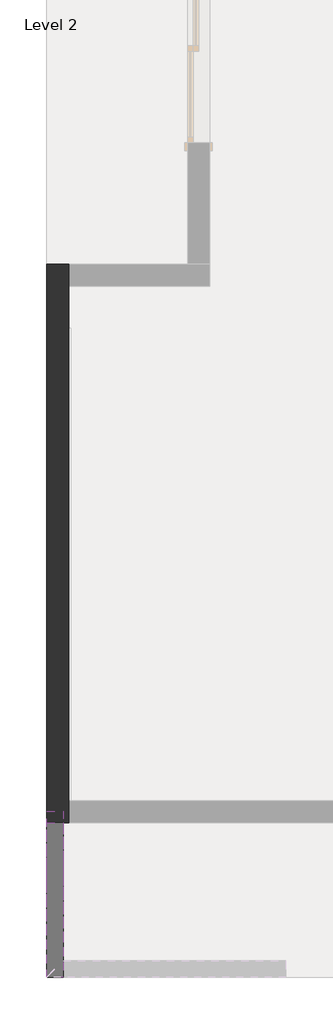
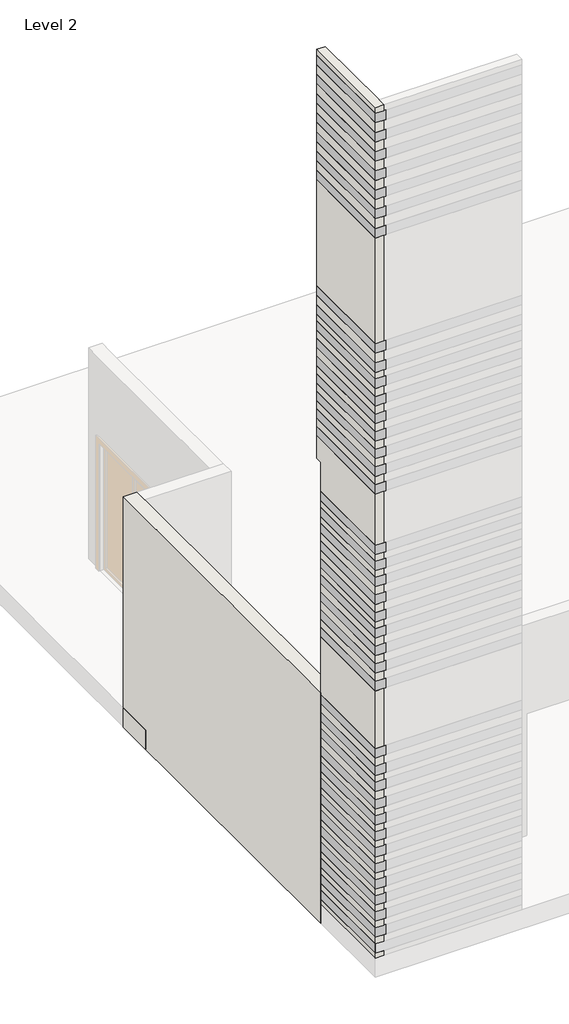
# One storey, part 1 of 2: 38 proxies, 2 walls.
"""IFC4 building model written with IfcOpenShell, lengths in millimetres."""

from ifc_helpers import new_model, si_unit, frame, origin, place, context, project, spatial, polyline, outline, extrude, faceted_brep, element, save

model = new_model("IFC4")

# Units and contexts
model_context = context("Model", 3, world=origin())
ifc_project = project(units=[si_unit("LENGTHUNIT", "METRE", prefix="MILLI")], contexts=[model_context])

# Site, building, storey
site = spatial("IfcSite", under=ifc_project)
building = spatial("IfcBuilding", under=site)
storey = spatial("IfcBuildingStorey", under=building, Name="Level 2", Elevation=3657.6)

# Proxies
placement = place(None, origin())
element("IfcBuildingElementProxy", 1, Name="Reveal", ObjectType="Reveal", at=placement, inside=storey, context=model_context, shape_type="SweptSolid", body=[
    extrude(outline(polyline([(-8860.5727738, -2566.8325754), (-8708.1727738, -2566.8325754), (-8708.1727738, -3836.8325754), (-8860.5727738, -3989.2325754), (-8860.5727738, -2566.8325754)])), frame((0.0, 0.0, 4038.6), z_axis=(0.0, 0.0, 1.0), x_axis=(1.0, 0.0, 0.0)), (0.0, 0.0, 1.0), 152.4),
])
element("IfcBuildingElementProxy", 2, Name="Reveal", ObjectType="Reveal", at=placement, inside=storey, context=model_context, shape_type="SweptSolid", body=[
    extrude(outline(polyline([(-8860.5727738, -2566.8325754), (-8708.1727738, -2566.8325754), (-8708.1727738, -3989.2325754), (-8860.5727738, -3989.2325754), (-8860.5727738, -2566.8325754)])), frame((0.0, 0.0, 4292.6), z_axis=(0.0, 0.0, 1.0), x_axis=(1.0, 0.0, 0.0)), (0.0, 0.0, 1.0), 152.4),
])
element("IfcBuildingElementProxy", 3, Name="Reveal", ObjectType="Reveal", at=placement, inside=storey, context=model_context, shape_type="SweptSolid", body=[
    extrude(outline(polyline([(-8860.5727738, -2566.8325754), (-8708.1727738, -2566.8325754), (-8708.1727738, -3989.2325754), (-8860.5727738, -3989.2325754), (-8860.5727738, -2566.8325754)])), frame((0.0, 0.0, 4546.6), z_axis=(0.0, 0.0, 1.0), x_axis=(1.0, 0.0, 0.0)), (0.0, 0.0, 1.0), 152.4),
])
element("IfcBuildingElementProxy", 4, Name="Reveal", ObjectType="Reveal", at=placement, inside=storey, context=model_context, shape_type="SweptSolid", body=[
    extrude(outline(polyline([(-8860.5727738, -2566.8325754), (-8708.1727738, -2566.8325754), (-8708.1727738, -3989.2325754), (-8860.5727738, -3989.2325754), (-8860.5727738, -2566.8325754)])), frame((0.0, 0.0, 4800.6), z_axis=(0.0, 0.0, 1.0), x_axis=(1.0, 0.0, 0.0)), (0.0, 0.0, 1.0), 152.4),
])
element("IfcBuildingElementProxy", 5, Name="Reveal", ObjectType="Reveal", at=placement, inside=storey, context=model_context, shape_type="SweptSolid", body=[
    extrude(outline(polyline([(-8860.5727738, -2566.8325754), (-8708.1727738, -2566.8325754), (-8708.1727738, -3989.2325754), (-8860.5727738, -3989.2325754), (-8860.5727738, -2566.8325754)])), frame((0.0, 0.0, 5054.6), z_axis=(0.0, 0.0, 1.0), x_axis=(1.0, 0.0, 0.0)), (0.0, 0.0, 1.0), 152.4),
])
element("IfcBuildingElementProxy", 6, Name="Reveal", ObjectType="Reveal", at=placement, inside=storey, context=model_context, shape_type="SweptSolid", body=[
    extrude(outline(polyline([(-8860.5727738, -2566.8325754), (-8708.1727738, -2566.8325754), (-8708.1727738, -3989.2325754), (-8860.5727738, -3989.2325754), (-8860.5727738, -2566.8325754)])), frame((0.0, 0.0, 5308.6), z_axis=(0.0, 0.0, 1.0), x_axis=(1.0, 0.0, 0.0)), (0.0, 0.0, 1.0), 152.4),
])
element("IfcBuildingElementProxy", 7, Name="Reveal", ObjectType="Reveal", at=placement, inside=storey, context=model_context, shape_type="SweptSolid", body=[
    extrude(outline(polyline([(-8860.5727738, -2566.8325754), (-8708.1727738, -2566.8325754), (-8708.1727738, -3989.2325754), (-8860.5727738, -3989.2325754), (-8860.5727738, -2566.8325754)])), frame((0.0, 0.0, 5562.6), z_axis=(0.0, 0.0, 1.0), x_axis=(1.0, 0.0, 0.0)), (0.0, 0.0, 1.0), 152.4),
])
element("IfcBuildingElementProxy", 8, Name="Reveal", ObjectType="Reveal", at=placement, inside=storey, context=model_context, shape_type="SweptSolid", body=[
    extrude(outline(polyline([(-8860.5727738, -2566.8325754), (-8708.1727738, -2566.8325754), (-8708.1727738, -3989.2325754), (-8860.5727738, -3989.2325754), (-8860.5727738, -2566.8325754)])), frame((0.0, 0.0, 5816.6), z_axis=(0.0, 0.0, 1.0), x_axis=(1.0, 0.0, 0.0)), (0.0, 0.0, 1.0), 152.4),
])
element("IfcBuildingElementProxy", 9, Name="Reveal", ObjectType="Reveal", at=placement, inside=storey, context=model_context, shape_type="SweptSolid", body=[
    extrude(outline(polyline([(-8860.5727738, -2566.8325754), (-8708.1727738, -2566.8325754), (-8708.1727738, -3989.2325754), (-8860.5727738, -3989.2325754), (-8860.5727738, -2566.8325754)])), frame((0.0, 0.0, 6070.6), z_axis=(0.0, 0.0, 1.0), x_axis=(1.0, 0.0, 0.0)), (0.0, 0.0, 1.0), 152.4),
])
element("IfcBuildingElementProxy", 10, Name="Reveal", ObjectType="Reveal", at=placement, inside=storey, context=model_context, shape_type="SweptSolid", body=[
    extrude(outline(polyline([(-8860.5727738, -2566.8325754), (-8708.1727738, -2566.8325754), (-8708.1727738, -3989.2325754), (-8860.5727738, -3989.2325754), (-8860.5727738, -2566.8325754)])), frame((0.0, 0.0, 6324.6), z_axis=(0.0, 0.0, 1.0), x_axis=(1.0, 0.0, 0.0)), (0.0, 0.0, 1.0), 152.4),
])
element("IfcBuildingElementProxy", 11, Name="Reveal", ObjectType="Reveal", at=placement, inside=storey, context=model_context, shape_type="SweptSolid", body=[
    extrude(outline(polyline([(-8860.5727738, -2566.8325754), (-8708.1727738, -2566.8325754), (-8708.1727738, -3989.2325754), (-8860.5727738, -3989.2325754), (-8860.5727738, -2566.8325754)])), frame((0.0, 0.0, 6604.0), z_axis=(0.0, 0.0, 1.0), x_axis=(1.0, 0.0, 0.0)), (0.0, 0.0, 1.0), 152.4),
])
element("IfcBuildingElementProxy", 12, Name="Reveal", ObjectType="Reveal", at=placement, inside=storey, context=model_context, shape_type="SweptSolid", body=[
    extrude(outline(polyline([(-8860.5727738, -2566.8325754), (-8708.1727738, -2566.8325754), (-8708.1727738, -3989.2325754), (-8860.5727738, -3989.2325754), (-8860.5727738, -2566.8325754)])), frame((0.0, 0.0, 6858.0), z_axis=(0.0, 0.0, 1.0), x_axis=(1.0, 0.0, 0.0)), (0.0, 0.0, 1.0), 152.4),
])
element("IfcBuildingElementProxy", 13, Name="Reveal", ObjectType="Reveal", at=placement, inside=storey, context=model_context, shape_type="SweptSolid", body=[
    extrude(outline(polyline([(-8860.5727738, -2566.8325754), (-8708.1727738, -2566.8325754), (-8708.1727738, -3989.2325754), (-8860.5727738, -3989.2325754), (-8860.5727738, -2566.8325754)])), frame((0.0, 0.0, 7137.4), z_axis=(0.0, 0.0, 1.0), x_axis=(1.0, 0.0, 0.0)), (0.0, 0.0, 1.0), 152.4),
])
element("IfcBuildingElementProxy", 14, Name="Reveal", ObjectType="Reveal", at=placement, inside=storey, context=model_context, shape_type="SweptSolid", body=[
    extrude(outline(polyline([(-8860.5727738, -2566.8325754), (-8708.1727738, -2566.8325754), (-8708.1727738, -3989.2325754), (-8860.5727738, -3989.2325754), (-8860.5727738, -2566.8325754)])), frame((0.0, 0.0, 8204.2), z_axis=(0.0, 0.0, 1.0), x_axis=(1.0, 0.0, 0.0)), (0.0, 0.0, 1.0), 152.4),
])
element("IfcBuildingElementProxy", 15, Name="Reveal", ObjectType="Reveal", at=placement, inside=storey, context=model_context, shape_type="SweptSolid", body=[
    extrude(outline(polyline([(-8860.5727738, -2566.8325754), (-8708.1727738, -2566.8325754), (-8708.1727738, -3989.2325754), (-8860.5727738, -3989.2325754), (-8860.5727738, -2566.8325754)])), frame((0.0, 0.0, 8483.6), z_axis=(0.0, 0.0, 1.0), x_axis=(1.0, 0.0, 0.0)), (0.0, 0.0, 1.0), 152.4),
])
element("IfcBuildingElementProxy", 16, Name="Reveal", ObjectType="Reveal", at=placement, inside=storey, context=model_context, shape_type="SweptSolid", body=[
    extrude(outline(polyline([(-8860.5727738, -2566.8325754), (-8708.1727738, -2566.8325754), (-8708.1727738, -3989.2325754), (-8860.5727738, -3989.2325754), (-8860.5727738, -2566.8325754)])), frame((0.0, 0.0, 8763.0), z_axis=(0.0, 0.0, 1.0), x_axis=(1.0, 0.0, 0.0)), (0.0, 0.0, 1.0), 152.4),
])
element("IfcBuildingElementProxy", 17, Name="Reveal", ObjectType="Reveal", at=placement, inside=storey, context=model_context, shape_type="SweptSolid", body=[
    extrude(outline(polyline([(-8860.5727738, -2566.8325754), (-8708.1727738, -2566.8325754), (-8708.1727738, -3989.2325754), (-8860.5727738, -3989.2325754), (-8860.5727738, -2566.8325754)])), frame((0.0, 0.0, 9042.4), z_axis=(0.0, 0.0, 1.0), x_axis=(1.0, 0.0, 0.0)), (0.0, 0.0, 1.0), 152.4),
])
element("IfcBuildingElementProxy", 18, Name="Reveal", ObjectType="Reveal", at=placement, inside=storey, context=model_context, shape_type="SweptSolid", body=[
    extrude(outline(polyline([(-8860.5727738, -2566.8325754), (-8708.1727738, -2566.8325754), (-8708.1727738, -3989.2325754), (-8860.5727738, -3989.2325754), (-8860.5727738, -2566.8325754)])), frame((0.0, 0.0, 9296.4), z_axis=(0.0, 0.0, 1.0), x_axis=(1.0, 0.0, 0.0)), (0.0, 0.0, 1.0), 152.4),
])
element("IfcBuildingElementProxy", 19, Name="Reveal", ObjectType="Reveal", at=placement, inside=storey, context=model_context, shape_type="SweptSolid", body=[
    extrude(outline(polyline([(-8860.5727738, -2566.8325754), (-8708.1727738, -2566.8325754), (-8708.1727738, -3989.2325754), (-8860.5727738, -3989.2325754), (-8860.5727738, -2566.8325754)])), frame((0.0, 0.0, 9575.8), z_axis=(0.0, 0.0, 1.0), x_axis=(1.0, 0.0, 0.0)), (0.0, 0.0, 1.0), 152.4),
])
element("IfcBuildingElementProxy", 20, Name="Reveal", ObjectType="Reveal", at=placement, inside=storey, context=model_context, shape_type="SweptSolid", body=[
    extrude(outline(polyline([(-8860.5727738, -2566.8325754), (-8708.1727738, -2566.8325754), (-8708.1727738, -3989.2325754), (-8860.5727738, -3989.2325754), (-8860.5727738, -2566.8325754)])), frame((0.0, 0.0, 9855.2), z_axis=(0.0, 0.0, 1.0), x_axis=(1.0, 0.0, 0.0)), (0.0, 0.0, 1.0), 152.4),
])
element("IfcBuildingElementProxy", 21, Name="Reveal", ObjectType="Reveal", at=placement, inside=storey, context=model_context, shape_type="SweptSolid", body=[
    extrude(outline(polyline([(-8860.5727738, -2566.8325754), (-8708.1727738, -2566.8325754), (-8708.1727738, -3989.2325754), (-8860.5727738, -3989.2325754), (-8860.5727738, -2566.8325754)])), frame((0.0, 0.0, 10109.2), z_axis=(0.0, 0.0, 1.0), x_axis=(1.0, 0.0, 0.0)), (0.0, 0.0, 1.0), 152.4),
])
element("IfcBuildingElementProxy", 22, Name="Reveal", ObjectType="Reveal", at=placement, inside=storey, context=model_context, shape_type="SweptSolid", body=[
    extrude(outline(polyline([(-8860.5727738, -2566.8325754), (-8708.1727738, -2566.8325754), (-8708.1727738, -3989.2325754), (-8860.5727738, -3989.2325754), (-8860.5727738, -2566.8325754)])), frame((0.0, 0.0, 10363.2), z_axis=(0.0, 0.0, 1.0), x_axis=(1.0, 0.0, 0.0)), (0.0, 0.0, 1.0), 152.4),
])
element("IfcBuildingElementProxy", 23, Name="Reveal", ObjectType="Reveal", at=placement, inside=storey, context=model_context, shape_type="SweptSolid", body=[
    extrude(outline(polyline([(-8860.5727738, -2465.2325754), (-8708.1727738, -2465.2325754), (-8708.1727738, -3989.2325754), (-8860.5727738, -3989.2325754), (-8860.5727738, -2465.2325754)])), frame((0.0, 0.0, 11328.4), z_axis=(0.0, 0.0, 1.0), x_axis=(1.0, 0.0, 0.0)), (0.0, 0.0, 1.0), 152.4),
])
element("IfcBuildingElementProxy", 24, Name="Reveal", ObjectType="Reveal", at=placement, inside=storey, context=model_context, shape_type="SweptSolid", body=[
    extrude(outline(polyline([(-8860.5727738, -2465.2325754), (-8708.1727738, -2465.2325754), (-8708.1727738, -3989.2325754), (-8860.5727738, -3989.2325754), (-8860.5727738, -2465.2325754)])), frame((0.0, 0.0, 11607.8), z_axis=(0.0, 0.0, 1.0), x_axis=(1.0, 0.0, 0.0)), (0.0, 0.0, 1.0), 152.4),
])
element("IfcBuildingElementProxy", 25, Name="Reveal", ObjectType="Reveal", at=placement, inside=storey, context=model_context, shape_type="SweptSolid", body=[
    extrude(outline(polyline([(-8860.5727738, -2465.2325754), (-8708.1727738, -2465.2325754), (-8708.1727738, -3989.2325754), (-8860.5727738, -3989.2325754), (-8860.5727738, -2465.2325754)])), frame((0.0, 0.0, 11887.2), z_axis=(0.0, 0.0, 1.0), x_axis=(1.0, 0.0, 0.0)), (0.0, 0.0, 1.0), 152.4),
])
element("IfcBuildingElementProxy", 26, Name="Reveal", ObjectType="Reveal", at=placement, inside=storey, context=model_context, shape_type="SweptSolid", body=[
    extrude(outline(polyline([(-8860.5727738, -2465.2325754), (-8708.1727738, -2465.2325754), (-8708.1727738, -3989.2325754), (-8860.5727738, -3989.2325754), (-8860.5727738, -2465.2325754)])), frame((0.0, 0.0, 12166.6), z_axis=(0.0, 0.0, 1.0), x_axis=(1.0, 0.0, 0.0)), (0.0, 0.0, 1.0), 152.4),
])
element("IfcBuildingElementProxy", 27, Name="Reveal", ObjectType="Reveal", at=placement, inside=storey, context=model_context, shape_type="SweptSolid", body=[
    extrude(outline(polyline([(-8860.5727738, -2465.2325754), (-8708.1727738, -2465.2325754), (-8708.1727738, -3989.2325754), (-8860.5727738, -3989.2325754), (-8860.5727738, -2465.2325754)])), frame((0.0, 0.0, 12446.0), z_axis=(0.0, 0.0, 1.0), x_axis=(1.0, 0.0, 0.0)), (0.0, 0.0, 1.0), 152.4),
])
element("IfcBuildingElementProxy", 28, Name="Reveal", ObjectType="Reveal", at=placement, inside=storey, context=model_context, shape_type="SweptSolid", body=[
    extrude(outline(polyline([(-8860.5727738, -2465.2325754), (-8708.1727738, -2465.2325754), (-8708.1727738, -3989.2325754), (-8860.5727738, -3989.2325754), (-8860.5727738, -2465.2325754)])), frame((0.0, 0.0, 12725.4), z_axis=(0.0, 0.0, 1.0), x_axis=(1.0, 0.0, 0.0)), (0.0, 0.0, 1.0), 152.4),
])
element("IfcBuildingElementProxy", 29, Name="Reveal", ObjectType="Reveal", at=placement, inside=storey, context=model_context, shape_type="SweptSolid", body=[
    extrude(outline(polyline([(-8860.5727738, -2465.2325754), (-8708.1727738, -2465.2325754), (-8708.1727738, -3989.2325754), (-8860.5727738, -3989.2325754), (-8860.5727738, -2465.2325754)])), frame((0.0, 0.0, 13004.8), z_axis=(0.0, 0.0, 1.0), x_axis=(1.0, 0.0, 0.0)), (0.0, 0.0, 1.0), 152.4),
])
element("IfcBuildingElementProxy", 30, Name="Reveal", ObjectType="Reveal", at=placement, inside=storey, context=model_context, shape_type="SweptSolid", body=[
    extrude(outline(polyline([(-8860.5727738, -2465.2325754), (-8708.1727738, -2465.2325754), (-8708.1727738, -3989.2325754), (-8860.5727738, -3989.2325754), (-8860.5727738, -2465.2325754)])), frame((0.0, 0.0, 13258.8), z_axis=(0.0, 0.0, 1.0), x_axis=(1.0, 0.0, 0.0)), (0.0, 0.0, 1.0), 152.4),
])
element("IfcBuildingElementProxy", 31, Name="Reveal", ObjectType="Reveal", at=placement, inside=storey, context=model_context, shape_type="SweptSolid", body=[
    extrude(outline(polyline([(-8860.5727738, -2465.2325754), (-8708.1727738, -2465.2325754), (-8708.1727738, -3989.2325754), (-8860.5727738, -3989.2325754), (-8860.5727738, -2465.2325754)])), frame((0.0, 0.0, 13563.6), z_axis=(0.0, 0.0, 1.0), x_axis=(1.0, 0.0, 0.0)), (0.0, 0.0, 1.0), 152.4),
])
element("IfcBuildingElementProxy", 32, Name="Reveal", ObjectType="Reveal", at=placement, inside=storey, context=model_context, shape_type="SweptSolid", body=[
    extrude(outline(polyline([(-8860.5727738, -2465.2325754), (-8708.1727738, -2465.2325754), (-8708.1727738, -3989.2325754), (-8860.5727738, -3989.2325754), (-8860.5727738, -2465.2325754)])), frame((0.0, 0.0, 15392.4), z_axis=(0.0, 0.0, 1.0), x_axis=(1.0, 0.0, 0.0)), (0.0, 0.0, 1.0), 152.4),
])
element("IfcBuildingElementProxy", 33, Name="Reveal", ObjectType="Reveal", at=placement, inside=storey, context=model_context, shape_type="SweptSolid", body=[
    extrude(outline(polyline([(-8860.5727738, -2465.2325754), (-8708.1727738, -2465.2325754), (-8708.1727738, -3989.2325754), (-8860.5727738, -3989.2325754), (-8860.5727738, -2465.2325754)])), frame((0.0, 0.0, 15697.2), z_axis=(0.0, 0.0, 1.0), x_axis=(1.0, 0.0, 0.0)), (0.0, 0.0, 1.0), 152.4),
])
element("IfcBuildingElementProxy", 34, Name="Reveal", ObjectType="Reveal", at=placement, inside=storey, context=model_context, shape_type="SweptSolid", body=[
    extrude(outline(polyline([(-8860.5727738, -2465.2325754), (-8708.1727738, -2465.2325754), (-8708.1727738, -3989.2325754), (-8860.5727738, -3989.2325754), (-8860.5727738, -2465.2325754)])), frame((0.0, 0.0, 16002.0), z_axis=(0.0, 0.0, 1.0), x_axis=(1.0, 0.0, 0.0)), (0.0, 0.0, 1.0), 152.4),
])
element("IfcBuildingElementProxy", 35, Name="Reveal", ObjectType="Reveal", at=placement, inside=storey, context=model_context, shape_type="SweptSolid", body=[
    extrude(outline(polyline([(-8860.5727738, -2465.2325754), (-8708.1727738, -2465.2325754), (-8708.1727738, -3989.2325754), (-8860.5727738, -3989.2325754), (-8860.5727738, -2465.2325754)])), frame((0.0, 0.0, 16306.8), z_axis=(0.0, 0.0, 1.0), x_axis=(1.0, 0.0, 0.0)), (0.0, 0.0, 1.0), 152.4),
])
element("IfcBuildingElementProxy", 36, Name="Reveal", ObjectType="Reveal", at=placement, inside=storey, context=model_context, shape_type="SweptSolid", body=[
    extrude(outline(polyline([(-8860.5727738, -2465.2325754), (-8708.1727738, -2465.2325754), (-8708.1727738, -3989.2325754), (-8860.5727738, -3989.2325754), (-8860.5727738, -2465.2325754)])), frame((0.0, 0.0, 16611.6), z_axis=(0.0, 0.0, 1.0), x_axis=(1.0, 0.0, 0.0)), (0.0, 0.0, 1.0), 152.4),
])
element("IfcBuildingElementProxy", 37, Name="Reveal", ObjectType="Reveal", at=placement, inside=storey, context=model_context, shape_type="SweptSolid", body=[
    extrude(outline(polyline([(-8860.5727738, -2465.2325754), (-8708.1727738, -2465.2325754), (-8708.1727738, -3989.2325754), (-8860.5727738, -3989.2325754), (-8860.5727738, -2465.2325754)])), frame((0.0, 0.0, 16916.4), z_axis=(0.0, 0.0, 1.0), x_axis=(1.0, 0.0, 0.0)), (0.0, 0.0, 1.0), 152.4),
])
element("IfcBuildingElementProxy", 38, Name="Reveal", ObjectType="Reveal", at=placement, inside=storey, context=model_context, shape_type="SweptSolid", body=[
    extrude(outline(polyline([(-8860.5727738, -2465.2325754), (-8708.1727738, -2465.2325754), (-8708.1727738, -3989.2325754), (-8860.5727738, -3989.2325754), (-8860.5727738, -2465.2325754)])), frame((0.0, 0.0, 17221.2), z_axis=(0.0, 0.0, 1.0), x_axis=(1.0, 0.0, 0.0)), (0.0, 0.0, 1.0), 152.4),
])

# Walls
element("IfcWall", 39, ObjectType="Generic - 5\"", at=placement, inside=storey, context=model_context, shape_type="Brep", body=[
    faceted_brep([(-8860.5727738, -2566.8325754, 3962.4), (-8860.5727738, -3989.2325754, 3962.4), (-8860.5727738, -3989.2325754, 4038.6), (-8860.5727738, -2566.8325754, 4038.6), (-8733.5727738, -3989.2325754, 3962.4), (-8733.5727738, -3862.2325754, 3962.4), (-8733.5727738, -2566.8325754, 3962.4), (-8733.5727738, -2566.8325754, 4038.6), (-8733.5727738, -3862.2325754, 4038.6), (-8733.5727738, -3989.2325754, 4038.6)], [[[0, 1, 2, 3]], [[4, 5, 6, 7, 8, 9]], [[1, 0, 6, 5, 4]], [[1, 4, 9, 2]], [[6, 0, 3, 7]], [[3, 2, 9, 8, 7]]]),
    faceted_brep([(-8860.5727738, -3989.2325754, 17464.824337), (-8860.5727738, -2465.2325754, 17464.824337), (-8860.5727738, -2465.2325754, 17373.6), (-8860.5727738, -3989.2325754, 17373.6), (-8733.5727738, -2465.2325754, 17464.824337), (-8733.5727738, -3862.2325754, 17464.824337), (-8733.5727738, -3989.2325754, 17464.824337), (-8733.5727738, -3989.2325754, 17373.6), (-8733.5727738, -3862.2325754, 17373.6), (-8733.5727738, -2465.2325754, 17373.6)], [[[0, 1, 2, 3]], [[4, 5, 6, 7, 8, 9]], [[1, 0, 6, 5, 4]], [[6, 0, 3, 7]], [[1, 4, 9, 2]], [[3, 2, 9, 8, 7]]]),
    faceted_brep([(-8860.5727738, -2465.2325754, 10972.8), (-8860.5727738, -2566.8325754, 10972.8), (-8860.5727738, -2566.8325754, 10515.6), (-8860.5727738, -3989.2325754, 10515.6), (-8860.5727738, -3989.2325754, 11328.4), (-8860.5727738, -2465.2325754, 11328.4), (-8733.5727738, -2566.8325754, 10972.8), (-8733.5727738, -2509.6825754, 10972.8), (-8733.5727738, -2465.2325754, 10972.8), (-8733.5727738, -2465.2325754, 11328.4), (-8733.5727738, -2509.6825754, 11328.4), (-8733.5727738, -3862.2325754, 11328.4), (-8733.5727738, -3989.2325754, 11328.4), (-8733.5727738, -3989.2325754, 10515.6), (-8733.5727738, -3862.2325754, 10515.6), (-8733.5727738, -2566.8325754, 10515.6)], [[[0, 1, 2, 3, 4, 5]], [[6, 7, 8, 9, 10, 11, 12, 13, 14, 15]], [[3, 13, 12, 4]], [[8, 0, 5, 9]], [[0, 8, 7, 6, 1]], [[1, 6, 15, 2]], [[3, 2, 15, 14, 13]], [[5, 4, 12, 11, 10, 9]]]),
    faceted_brep([(-8860.5727738, -2566.8325754, 4191.0), (-8860.5727738, -3989.2325754, 4191.0), (-8860.5727738, -3989.2325754, 4292.6), (-8860.5727738, -2566.8325754, 4292.6), (-8733.5727738, -3989.2325754, 4191.0), (-8733.5727738, -3862.2325754, 4191.0), (-8733.5727738, -2566.8325754, 4191.0), (-8733.5727738, -2566.8325754, 4292.6), (-8733.5727738, -3862.2325754, 4292.6), (-8733.5727738, -3989.2325754, 4292.6)], [[[0, 1, 2, 3]], [[4, 5, 6, 7, 8, 9]], [[1, 4, 9, 2]], [[6, 0, 3, 7]], [[1, 0, 6, 5, 4]], [[3, 2, 9, 8, 7]]]),
    faceted_brep([(-8860.5727738, -2566.8325754, 4445.0), (-8860.5727738, -3989.2325754, 4445.0), (-8860.5727738, -3989.2325754, 4546.6), (-8860.5727738, -2566.8325754, 4546.6), (-8733.5727738, -3989.2325754, 4445.0), (-8733.5727738, -3862.2325754, 4445.0), (-8733.5727738, -2566.8325754, 4445.0), (-8733.5727738, -2566.8325754, 4546.6), (-8733.5727738, -3862.2325754, 4546.6), (-8733.5727738, -3989.2325754, 4546.6)], [[[0, 1, 2, 3]], [[4, 5, 6, 7, 8, 9]], [[1, 4, 9, 2]], [[6, 0, 3, 7]], [[1, 0, 6, 5, 4]], [[3, 2, 9, 8, 7]]]),
    faceted_brep([(-8860.5727738, -2566.8325754, 4699.0), (-8860.5727738, -3989.2325754, 4699.0), (-8860.5727738, -3989.2325754, 4800.6), (-8860.5727738, -2566.8325754, 4800.6), (-8733.5727738, -3989.2325754, 4699.0), (-8733.5727738, -3862.2325754, 4699.0), (-8733.5727738, -2566.8325754, 4699.0), (-8733.5727738, -2566.8325754, 4800.6), (-8733.5727738, -3862.2325754, 4800.6), (-8733.5727738, -3989.2325754, 4800.6)], [[[0, 1, 2, 3]], [[4, 5, 6, 7, 8, 9]], [[1, 4, 9, 2]], [[6, 0, 3, 7]], [[1, 0, 6, 5, 4]], [[3, 2, 9, 8, 7]]]),
    faceted_brep([(-8860.5727738, -2566.8325754, 4953.0), (-8860.5727738, -3989.2325754, 4953.0), (-8860.5727738, -3989.2325754, 5054.6), (-8860.5727738, -2566.8325754, 5054.6), (-8733.5727738, -3989.2325754, 4953.0), (-8733.5727738, -3862.2325754, 4953.0), (-8733.5727738, -2566.8325754, 4953.0), (-8733.5727738, -2566.8325754, 5054.6), (-8733.5727738, -3862.2325754, 5054.6), (-8733.5727738, -3989.2325754, 5054.6)], [[[0, 1, 2, 3]], [[4, 5, 6, 7, 8, 9]], [[1, 4, 9, 2]], [[6, 0, 3, 7]], [[1, 0, 6, 5, 4]], [[3, 2, 9, 8, 7]]]),
    faceted_brep([(-8860.5727738, -2566.8325754, 5207.0), (-8860.5727738, -3989.2325754, 5207.0), (-8860.5727738, -3989.2325754, 5308.6), (-8860.5727738, -2566.8325754, 5308.6), (-8733.5727738, -3989.2325754, 5207.0), (-8733.5727738, -3862.2325754, 5207.0), (-8733.5727738, -2566.8325754, 5207.0), (-8733.5727738, -2566.8325754, 5308.6), (-8733.5727738, -3862.2325754, 5308.6), (-8733.5727738, -3989.2325754, 5308.6)], [[[0, 1, 2, 3]], [[4, 5, 6, 7, 8, 9]], [[1, 4, 9, 2]], [[6, 0, 3, 7]], [[1, 0, 6, 5, 4]], [[3, 2, 9, 8, 7]]]),
    faceted_brep([(-8860.5727738, -2566.8325754, 5461.0), (-8860.5727738, -3989.2325754, 5461.0), (-8860.5727738, -3989.2325754, 5562.6), (-8860.5727738, -2566.8325754, 5562.6), (-8733.5727738, -3989.2325754, 5461.0), (-8733.5727738, -3862.2325754, 5461.0), (-8733.5727738, -2566.8325754, 5461.0), (-8733.5727738, -2566.8325754, 5562.6), (-8733.5727738, -3862.2325754, 5562.6), (-8733.5727738, -3989.2325754, 5562.6)], [[[0, 1, 2, 3]], [[4, 5, 6, 7, 8, 9]], [[1, 4, 9, 2]], [[6, 0, 3, 7]], [[1, 0, 6, 5, 4]], [[3, 2, 9, 8, 7]]]),
    faceted_brep([(-8860.5727738, -2566.8325754, 5715.0), (-8860.5727738, -3989.2325754, 5715.0), (-8860.5727738, -3989.2325754, 5816.6), (-8860.5727738, -2566.8325754, 5816.6), (-8733.5727738, -3989.2325754, 5715.0), (-8733.5727738, -3862.2325754, 5715.0), (-8733.5727738, -2566.8325754, 5715.0), (-8733.5727738, -2566.8325754, 5816.6), (-8733.5727738, -3862.2325754, 5816.6), (-8733.5727738, -3989.2325754, 5816.6)], [[[0, 1, 2, 3]], [[4, 5, 6, 7, 8, 9]], [[1, 4, 9, 2]], [[6, 0, 3, 7]], [[1, 0, 6, 5, 4]], [[3, 2, 9, 8, 7]]]),
    faceted_brep([(-8860.5727738, -2566.8325754, 5969.0), (-8860.5727738, -3989.2325754, 5969.0), (-8860.5727738, -3989.2325754, 6070.6), (-8860.5727738, -2566.8325754, 6070.6), (-8733.5727738, -3989.2325754, 5969.0), (-8733.5727738, -3862.2325754, 5969.0), (-8733.5727738, -2566.8325754, 5969.0), (-8733.5727738, -2566.8325754, 6070.6), (-8733.5727738, -3862.2325754, 6070.6), (-8733.5727738, -3989.2325754, 6070.6)], [[[0, 1, 2, 3]], [[4, 5, 6, 7, 8, 9]], [[1, 4, 9, 2]], [[6, 0, 3, 7]], [[1, 0, 6, 5, 4]], [[3, 2, 9, 8, 7]]]),
    faceted_brep([(-8860.5727738, -2566.8325754, 6223.0), (-8860.5727738, -3989.2325754, 6223.0), (-8860.5727738, -3989.2325754, 6324.6), (-8860.5727738, -2566.8325754, 6324.6), (-8733.5727738, -3989.2325754, 6223.0), (-8733.5727738, -3862.2325754, 6223.0), (-8733.5727738, -2566.8325754, 6223.0), (-8733.5727738, -2566.8325754, 6324.6), (-8733.5727738, -3862.2325754, 6324.6), (-8733.5727738, -3989.2325754, 6324.6)], [[[0, 1, 2, 3]], [[4, 5, 6, 7, 8, 9]], [[1, 4, 9, 2]], [[6, 0, 3, 7]], [[1, 0, 6, 5, 4]], [[3, 2, 9, 8, 7]]]),
    faceted_brep([(-8860.5727738, -2566.8325754, 6477.0), (-8860.5727738, -3989.2325754, 6477.0), (-8860.5727738, -3989.2325754, 6604.0), (-8860.5727738, -2566.8325754, 6604.0), (-8733.5727738, -3989.2325754, 6477.0), (-8733.5727738, -3862.2325754, 6477.0), (-8733.5727738, -2566.8325754, 6477.0), (-8733.5727738, -2566.8325754, 6604.0), (-8733.5727738, -3862.2325754, 6604.0), (-8733.5727738, -3989.2325754, 6604.0)], [[[0, 1, 2, 3]], [[4, 5, 6, 7, 8, 9]], [[1, 4, 9, 2]], [[6, 0, 3, 7]], [[1, 0, 6, 5, 4]], [[3, 2, 9, 8, 7]]]),
    faceted_brep([(-8860.5727738, -2566.8325754, 6756.4), (-8860.5727738, -3989.2325754, 6756.4), (-8860.5727738, -3989.2325754, 6858.0), (-8860.5727738, -2566.8325754, 6858.0), (-8733.5727738, -3989.2325754, 6756.4), (-8733.5727738, -3862.2325754, 6756.4), (-8733.5727738, -2566.8325754, 6756.4), (-8733.5727738, -2566.8325754, 6858.0), (-8733.5727738, -3862.2325754, 6858.0), (-8733.5727738, -3989.2325754, 6858.0)], [[[0, 1, 2, 3]], [[4, 5, 6, 7, 8, 9]], [[1, 4, 9, 2]], [[6, 0, 3, 7]], [[1, 0, 6, 5, 4]], [[3, 2, 9, 8, 7]]]),
    faceted_brep([(-8860.5727738, -2566.8325754, 7010.4), (-8860.5727738, -3989.2325754, 7010.4), (-8860.5727738, -3989.2325754, 7137.4), (-8860.5727738, -2566.8325754, 7137.4), (-8733.5727738, -3989.2325754, 7010.4), (-8733.5727738, -3862.2325754, 7010.4), (-8733.5727738, -2566.8325754, 7010.4), (-8733.5727738, -2566.8325754, 7137.4), (-8733.5727738, -3862.2325754, 7137.4), (-8733.5727738, -3989.2325754, 7137.4)], [[[0, 1, 2, 3]], [[4, 5, 6, 7, 8, 9]], [[1, 4, 9, 2]], [[6, 0, 3, 7]], [[1, 0, 6, 5, 4]], [[3, 2, 9, 8, 7]]]),
    faceted_brep([(-8860.5727738, -2566.8325754, 7289.8), (-8860.5727738, -3989.2325754, 7289.8), (-8860.5727738, -3989.2325754, 8204.2), (-8860.5727738, -2566.8325754, 8204.2), (-8860.5727738, -2566.8325754, 7315.2), (-8733.5727738, -3989.2325754, 7289.8), (-8733.5727738, -3862.2325754, 7289.8), (-8733.5727738, -2566.8325754, 7289.8), (-8733.5727738, -2566.8325754, 8204.2), (-8733.5727738, -3862.2325754, 8204.2), (-8733.5727738, -3989.2325754, 8204.2)], [[[0, 1, 2, 3, 4]], [[5, 6, 7, 8, 9, 10]], [[1, 5, 10, 2]], [[7, 0, 4, 3, 8]], [[1, 0, 7, 6, 5]], [[3, 2, 10, 9, 8]]]),
    faceted_brep([(-8860.5727738, -2566.8325754, 8356.6), (-8860.5727738, -3989.2325754, 8356.6), (-8860.5727738, -3989.2325754, 8483.6), (-8860.5727738, -2566.8325754, 8483.6), (-8733.5727738, -3989.2325754, 8356.6), (-8733.5727738, -3862.2325754, 8356.6), (-8733.5727738, -2566.8325754, 8356.6), (-8733.5727738, -2566.8325754, 8483.6), (-8733.5727738, -3862.2325754, 8483.6), (-8733.5727738, -3989.2325754, 8483.6)], [[[0, 1, 2, 3]], [[4, 5, 6, 7, 8, 9]], [[1, 4, 9, 2]], [[6, 0, 3, 7]], [[1, 0, 6, 5, 4]], [[3, 2, 9, 8, 7]]]),
    faceted_brep([(-8860.5727738, -2566.8325754, 8636.0), (-8860.5727738, -3989.2325754, 8636.0), (-8860.5727738, -3989.2325754, 8763.0), (-8860.5727738, -2566.8325754, 8763.0), (-8733.5727738, -3989.2325754, 8636.0), (-8733.5727738, -3862.2325754, 8636.0), (-8733.5727738, -2566.8325754, 8636.0), (-8733.5727738, -2566.8325754, 8763.0), (-8733.5727738, -3862.2325754, 8763.0), (-8733.5727738, -3989.2325754, 8763.0)], [[[0, 1, 2, 3]], [[4, 5, 6, 7, 8, 9]], [[1, 4, 9, 2]], [[6, 0, 3, 7]], [[1, 0, 6, 5, 4]], [[3, 2, 9, 8, 7]]]),
    faceted_brep([(-8860.5727738, -2566.8325754, 8915.4), (-8860.5727738, -3989.2325754, 8915.4), (-8860.5727738, -3989.2325754, 9042.4), (-8860.5727738, -2566.8325754, 9042.4), (-8733.5727738, -3989.2325754, 8915.4), (-8733.5727738, -3862.2325754, 8915.4), (-8733.5727738, -2566.8325754, 8915.4), (-8733.5727738, -2566.8325754, 9042.4), (-8733.5727738, -3862.2325754, 9042.4), (-8733.5727738, -3989.2325754, 9042.4)], [[[0, 1, 2, 3]], [[4, 5, 6, 7, 8, 9]], [[1, 4, 9, 2]], [[6, 0, 3, 7]], [[1, 0, 6, 5, 4]], [[3, 2, 9, 8, 7]]]),
    faceted_brep([(-8860.5727738, -2566.8325754, 9194.8), (-8860.5727738, -3989.2325754, 9194.8), (-8860.5727738, -3989.2325754, 9296.4), (-8860.5727738, -2566.8325754, 9296.4), (-8733.5727738, -3989.2325754, 9194.8), (-8733.5727738, -3862.2325754, 9194.8), (-8733.5727738, -2566.8325754, 9194.8), (-8733.5727738, -2566.8325754, 9296.4), (-8733.5727738, -3862.2325754, 9296.4), (-8733.5727738, -3989.2325754, 9296.4)], [[[0, 1, 2, 3]], [[4, 5, 6, 7, 8, 9]], [[1, 4, 9, 2]], [[6, 0, 3, 7]], [[1, 0, 6, 5, 4]], [[3, 2, 9, 8, 7]]]),
    faceted_brep([(-8860.5727738, -2566.8325754, 9448.8), (-8860.5727738, -3989.2325754, 9448.8), (-8860.5727738, -3989.2325754, 9575.8), (-8860.5727738, -2566.8325754, 9575.8), (-8733.5727738, -3989.2325754, 9448.8), (-8733.5727738, -3862.2325754, 9448.8), (-8733.5727738, -2566.8325754, 9448.8), (-8733.5727738, -2566.8325754, 9575.8), (-8733.5727738, -3862.2325754, 9575.8), (-8733.5727738, -3989.2325754, 9575.8)], [[[0, 1, 2, 3]], [[4, 5, 6, 7, 8, 9]], [[1, 4, 9, 2]], [[6, 0, 3, 7]], [[1, 0, 6, 5, 4]], [[3, 2, 9, 8, 7]]]),
    faceted_brep([(-8860.5727738, -2566.8325754, 9728.2), (-8860.5727738, -3989.2325754, 9728.2), (-8860.5727738, -3989.2325754, 9855.2), (-8860.5727738, -2566.8325754, 9855.2), (-8733.5727738, -3989.2325754, 9728.2), (-8733.5727738, -3862.2325754, 9728.2), (-8733.5727738, -2566.8325754, 9728.2), (-8733.5727738, -2566.8325754, 9855.2), (-8733.5727738, -3862.2325754, 9855.2), (-8733.5727738, -3989.2325754, 9855.2)], [[[0, 1, 2, 3]], [[4, 5, 6, 7, 8, 9]], [[1, 4, 9, 2]], [[6, 0, 3, 7]], [[1, 0, 6, 5, 4]], [[3, 2, 9, 8, 7]]]),
    faceted_brep([(-8860.5727738, -2566.8325754, 10007.6), (-8860.5727738, -3989.2325754, 10007.6), (-8860.5727738, -3989.2325754, 10109.2), (-8860.5727738, -2566.8325754, 10109.2), (-8733.5727738, -3989.2325754, 10007.6), (-8733.5727738, -3862.2325754, 10007.6), (-8733.5727738, -2566.8325754, 10007.6), (-8733.5727738, -2566.8325754, 10109.2), (-8733.5727738, -3862.2325754, 10109.2), (-8733.5727738, -3989.2325754, 10109.2)], [[[0, 1, 2, 3]], [[4, 5, 6, 7, 8, 9]], [[1, 4, 9, 2]], [[6, 0, 3, 7]], [[1, 0, 6, 5, 4]], [[3, 2, 9, 8, 7]]]),
    faceted_brep([(-8860.5727738, -2566.8325754, 10261.6), (-8860.5727738, -3989.2325754, 10261.6), (-8860.5727738, -3989.2325754, 10363.2), (-8860.5727738, -2566.8325754, 10363.2), (-8733.5727738, -3989.2325754, 10261.6), (-8733.5727738, -3862.2325754, 10261.6), (-8733.5727738, -2566.8325754, 10261.6), (-8733.5727738, -2566.8325754, 10363.2), (-8733.5727738, -3862.2325754, 10363.2), (-8733.5727738, -3989.2325754, 10363.2)], [[[0, 1, 2, 3]], [[4, 5, 6, 7, 8, 9]], [[1, 4, 9, 2]], [[6, 0, 3, 7]], [[1, 0, 6, 5, 4]], [[3, 2, 9, 8, 7]]]),
    faceted_brep([(-8860.5727738, -2465.2325754, 11480.8), (-8860.5727738, -3989.2325754, 11480.8), (-8860.5727738, -3989.2325754, 11607.8), (-8860.5727738, -2465.2325754, 11607.8), (-8733.5727738, -3989.2325754, 11480.8), (-8733.5727738, -3862.2325754, 11480.8), (-8733.5727738, -2509.6825754, 11480.8), (-8733.5727738, -2465.2325754, 11480.8), (-8733.5727738, -2465.2325754, 11607.8), (-8733.5727738, -2509.6825754, 11607.8), (-8733.5727738, -3862.2325754, 11607.8), (-8733.5727738, -3989.2325754, 11607.8)], [[[0, 1, 2, 3]], [[4, 5, 6, 7, 8, 9, 10, 11]], [[1, 4, 11, 2]], [[7, 0, 3, 8]], [[1, 0, 7, 6, 5, 4]], [[3, 2, 11, 10, 9, 8]]]),
    faceted_brep([(-8860.5727738, -2465.2325754, 11760.2), (-8860.5727738, -3989.2325754, 11760.2), (-8860.5727738, -3989.2325754, 11887.2), (-8860.5727738, -2465.2325754, 11887.2), (-8733.5727738, -3989.2325754, 11760.2), (-8733.5727738, -3862.2325754, 11760.2), (-8733.5727738, -2509.6825754, 11760.2), (-8733.5727738, -2465.2325754, 11760.2), (-8733.5727738, -2465.2325754, 11887.2), (-8733.5727738, -2509.6825754, 11887.2), (-8733.5727738, -3862.2325754, 11887.2), (-8733.5727738, -3989.2325754, 11887.2)], [[[0, 1, 2, 3]], [[4, 5, 6, 7, 8, 9, 10, 11]], [[1, 4, 11, 2]], [[7, 0, 3, 8]], [[1, 0, 7, 6, 5, 4]], [[3, 2, 11, 10, 9, 8]]]),
    faceted_brep([(-8860.5727738, -2465.2325754, 12039.6), (-8860.5727738, -3989.2325754, 12039.6), (-8860.5727738, -3989.2325754, 12166.6), (-8860.5727738, -2465.2325754, 12166.6), (-8733.5727738, -3989.2325754, 12039.6), (-8733.5727738, -3862.2325754, 12039.6), (-8733.5727738, -2509.6825754, 12039.6), (-8733.5727738, -2465.2325754, 12039.6), (-8733.5727738, -2465.2325754, 12166.6), (-8733.5727738, -2509.6825754, 12166.6), (-8733.5727738, -3862.2325754, 12166.6), (-8733.5727738, -3989.2325754, 12166.6)], [[[0, 1, 2, 3]], [[4, 5, 6, 7, 8, 9, 10, 11]], [[1, 4, 11, 2]], [[7, 0, 3, 8]], [[1, 0, 7, 6, 5, 4]], [[3, 2, 11, 10, 9, 8]]]),
    faceted_brep([(-8860.5727738, -2465.2325754, 12319.0), (-8860.5727738, -3989.2325754, 12319.0), (-8860.5727738, -3989.2325754, 12446.0), (-8860.5727738, -2465.2325754, 12446.0), (-8733.5727738, -3989.2325754, 12319.0), (-8733.5727738, -3862.2325754, 12319.0), (-8733.5727738, -2509.6825754, 12319.0), (-8733.5727738, -2465.2325754, 12319.0), (-8733.5727738, -2465.2325754, 12446.0), (-8733.5727738, -2509.6825754, 12446.0), (-8733.5727738, -3862.2325754, 12446.0), (-8733.5727738, -3989.2325754, 12446.0)], [[[0, 1, 2, 3]], [[4, 5, 6, 7, 8, 9, 10, 11]], [[1, 4, 11, 2]], [[7, 0, 3, 8]], [[1, 0, 7, 6, 5, 4]], [[3, 2, 11, 10, 9, 8]]]),
    faceted_brep([(-8860.5727738, -2465.2325754, 12598.4), (-8860.5727738, -3989.2325754, 12598.4), (-8860.5727738, -3989.2325754, 12725.4), (-8860.5727738, -2465.2325754, 12725.4), (-8733.5727738, -3989.2325754, 12598.4), (-8733.5727738, -3862.2325754, 12598.4), (-8733.5727738, -2509.6825754, 12598.4), (-8733.5727738, -2465.2325754, 12598.4), (-8733.5727738, -2465.2325754, 12725.4), (-8733.5727738, -2509.6825754, 12725.4), (-8733.5727738, -3862.2325754, 12725.4), (-8733.5727738, -3989.2325754, 12725.4)], [[[0, 1, 2, 3]], [[4, 5, 6, 7, 8, 9, 10, 11]], [[1, 4, 11, 2]], [[7, 0, 3, 8]], [[1, 0, 7, 6, 5, 4]], [[3, 2, 11, 10, 9, 8]]]),
    faceted_brep([(-8860.5727738, -2465.2325754, 12877.8), (-8860.5727738, -3989.2325754, 12877.8), (-8860.5727738, -3989.2325754, 13004.8), (-8860.5727738, -2465.2325754, 13004.8), (-8733.5727738, -3989.2325754, 12877.8), (-8733.5727738, -3862.2325754, 12877.8), (-8733.5727738, -2509.6825754, 12877.8), (-8733.5727738, -2465.2325754, 12877.8), (-8733.5727738, -2465.2325754, 13004.8), (-8733.5727738, -2509.6825754, 13004.8), (-8733.5727738, -3862.2325754, 13004.8), (-8733.5727738, -3989.2325754, 13004.8)], [[[0, 1, 2, 3]], [[4, 5, 6, 7, 8, 9, 10, 11]], [[1, 4, 11, 2]], [[7, 0, 3, 8]], [[1, 0, 7, 6, 5, 4]], [[3, 2, 11, 10, 9, 8]]]),
    faceted_brep([(-8860.5727738, -2465.2325754, 13157.2), (-8860.5727738, -3989.2325754, 13157.2), (-8860.5727738, -3989.2325754, 13258.8), (-8860.5727738, -2465.2325754, 13258.8), (-8733.5727738, -3989.2325754, 13157.2), (-8733.5727738, -3862.2325754, 13157.2), (-8733.5727738, -2509.6825754, 13157.2), (-8733.5727738, -2465.2325754, 13157.2), (-8733.5727738, -2465.2325754, 13258.8), (-8733.5727738, -2509.6825754, 13258.8), (-8733.5727738, -3862.2325754, 13258.8), (-8733.5727738, -3989.2325754, 13258.8)], [[[0, 1, 2, 3]], [[4, 5, 6, 7, 8, 9, 10, 11]], [[1, 4, 11, 2]], [[7, 0, 3, 8]], [[1, 0, 7, 6, 5, 4]], [[3, 2, 11, 10, 9, 8]]]),
    faceted_brep([(-8860.5727738, -2465.2325754, 13411.2), (-8860.5727738, -3989.2325754, 13411.2), (-8860.5727738, -3989.2325754, 13563.6), (-8860.5727738, -2465.2325754, 13563.6), (-8733.5727738, -3989.2325754, 13411.2), (-8733.5727738, -3862.2325754, 13411.2), (-8733.5727738, -2509.6825754, 13411.2), (-8733.5727738, -2465.2325754, 13411.2), (-8733.5727738, -2465.2325754, 13563.6), (-8733.5727738, -2509.6825754, 13563.6), (-8733.5727738, -3862.2325754, 13563.6), (-8733.5727738, -3989.2325754, 13563.6)], [[[0, 1, 2, 3]], [[4, 5, 6, 7, 8, 9, 10, 11]], [[1, 4, 11, 2]], [[7, 0, 3, 8]], [[1, 0, 7, 6, 5, 4]], [[3, 2, 11, 10, 9, 8]]]),
    faceted_brep([(-8860.5727738, -2465.2325754, 13716.0), (-8860.5727738, -3989.2325754, 13716.0), (-8860.5727738, -3989.2325754, 15392.4), (-8860.5727738, -2465.2325754, 15392.4), (-8860.5727738, -2465.2325754, 14630.4), (-8733.5727738, -3989.2325754, 13716.0), (-8733.5727738, -3862.2325754, 13716.0), (-8733.5727738, -2509.6825754, 13716.0), (-8733.5727738, -2465.2325754, 13716.0), (-8733.5727738, -2465.2325754, 14630.4), (-8733.5727738, -2465.2325754, 15392.4), (-8733.5727738, -3862.2325754, 15392.4), (-8733.5727738, -3989.2325754, 15392.4)], [[[0, 1, 2, 3, 4]], [[5, 6, 7, 8, 9, 10, 11, 12]], [[1, 5, 12, 2]], [[8, 0, 4, 3, 10, 9]], [[1, 0, 8, 7, 6, 5]], [[3, 2, 12, 11, 10]]]),
    faceted_brep([(-8860.5727738, -2465.2325754, 15544.8), (-8860.5727738, -3989.2325754, 15544.8), (-8860.5727738, -3989.2325754, 15697.2), (-8860.5727738, -2465.2325754, 15697.2), (-8733.5727738, -3989.2325754, 15544.8), (-8733.5727738, -3862.2325754, 15544.8), (-8733.5727738, -2465.2325754, 15544.8), (-8733.5727738, -2465.2325754, 15697.2), (-8733.5727738, -3862.2325754, 15697.2), (-8733.5727738, -3989.2325754, 15697.2)], [[[0, 1, 2, 3]], [[4, 5, 6, 7, 8, 9]], [[1, 4, 9, 2]], [[6, 0, 3, 7]], [[1, 0, 6, 5, 4]], [[3, 2, 9, 8, 7]]]),
    faceted_brep([(-8860.5727738, -2465.2325754, 15849.6), (-8860.5727738, -3989.2325754, 15849.6), (-8860.5727738, -3989.2325754, 16002.0), (-8860.5727738, -2465.2325754, 16002.0), (-8733.5727738, -3989.2325754, 15849.6), (-8733.5727738, -3862.2325754, 15849.6), (-8733.5727738, -2465.2325754, 15849.6), (-8733.5727738, -2465.2325754, 16002.0), (-8733.5727738, -3862.2325754, 16002.0), (-8733.5727738, -3989.2325754, 16002.0)], [[[0, 1, 2, 3]], [[4, 5, 6, 7, 8, 9]], [[1, 4, 9, 2]], [[6, 0, 3, 7]], [[1, 0, 6, 5, 4]], [[3, 2, 9, 8, 7]]]),
    faceted_brep([(-8860.5727738, -2465.2325754, 16154.4), (-8860.5727738, -3989.2325754, 16154.4), (-8860.5727738, -3989.2325754, 16306.8), (-8860.5727738, -2465.2325754, 16306.8), (-8733.5727738, -3989.2325754, 16154.4), (-8733.5727738, -3862.2325754, 16154.4), (-8733.5727738, -2465.2325754, 16154.4), (-8733.5727738, -2465.2325754, 16306.8), (-8733.5727738, -3862.2325754, 16306.8), (-8733.5727738, -3989.2325754, 16306.8)], [[[0, 1, 2, 3]], [[4, 5, 6, 7, 8, 9]], [[1, 4, 9, 2]], [[6, 0, 3, 7]], [[1, 0, 6, 5, 4]], [[3, 2, 9, 8, 7]]]),
    faceted_brep([(-8860.5727738, -2465.2325754, 16459.2), (-8860.5727738, -3989.2325754, 16459.2), (-8860.5727738, -3989.2325754, 16611.6), (-8860.5727738, -2465.2325754, 16611.6), (-8733.5727738, -3989.2325754, 16459.2), (-8733.5727738, -3862.2325754, 16459.2), (-8733.5727738, -2465.2325754, 16459.2), (-8733.5727738, -2465.2325754, 16611.6), (-8733.5727738, -3862.2325754, 16611.6), (-8733.5727738, -3989.2325754, 16611.6)], [[[0, 1, 2, 3]], [[4, 5, 6, 7, 8, 9]], [[1, 4, 9, 2]], [[6, 0, 3, 7]], [[1, 0, 6, 5, 4]], [[3, 2, 9, 8, 7]]]),
    faceted_brep([(-8860.5727738, -2465.2325754, 16764.0), (-8860.5727738, -3989.2325754, 16764.0), (-8860.5727738, -3989.2325754, 16916.4), (-8860.5727738, -2465.2325754, 16916.4), (-8733.5727738, -3989.2325754, 16764.0), (-8733.5727738, -3862.2325754, 16764.0), (-8733.5727738, -2465.2325754, 16764.0), (-8733.5727738, -2465.2325754, 16916.4), (-8733.5727738, -3862.2325754, 16916.4), (-8733.5727738, -3989.2325754, 16916.4)], [[[0, 1, 2, 3]], [[4, 5, 6, 7, 8, 9]], [[1, 4, 9, 2]], [[6, 0, 3, 7]], [[1, 0, 6, 5, 4]], [[3, 2, 9, 8, 7]]]),
    faceted_brep([(-8860.5727738, -2465.2325754, 17068.8), (-8860.5727738, -3989.2325754, 17068.8), (-8860.5727738, -3989.2325754, 17221.2), (-8860.5727738, -2465.2325754, 17221.2), (-8733.5727738, -3989.2325754, 17068.8), (-8733.5727738, -3862.2325754, 17068.8), (-8733.5727738, -2465.2325754, 17068.8), (-8733.5727738, -2465.2325754, 17221.2), (-8733.5727738, -3862.2325754, 17221.2), (-8733.5727738, -3989.2325754, 17221.2)], [[[0, 1, 2, 3]], [[4, 5, 6, 7, 8, 9]], [[1, 4, 9, 2]], [[6, 0, 3, 7]], [[1, 0, 6, 5, 4]], [[3, 2, 9, 8, 7]]]),
])
element("IfcWall", 40, ObjectType="Generic - 8\"", at=placement, inside=storey, context=model_context, shape_type="Brep", body=[
    faceted_brep([(-8657.3727738, -2566.8325754, 7315.2), (-8657.3727738, -2566.8325754, 3657.6), (-8657.3727738, -2363.6325754, 3657.6), (-8657.3727738, 2360.7674246, 3657.6), (-8657.3727738, 2563.9674246, 3657.6), (-8657.3727738, 2563.9674246, 7315.2), (-8657.3727738, 2360.7674246, 7315.2), (-8657.3727738, -2363.6325754, 7315.2), (-8860.5727738, -2566.8325754, 3657.6), (-8860.5727738, -2566.8325754, 3962.4), (-8860.5727738, -2566.8325754, 4038.6), (-8860.5727738, -2566.8325754, 4191.0), (-8860.5727738, -2566.8325754, 4292.6), (-8860.5727738, -2566.8325754, 4445.0), (-8860.5727738, -2566.8325754, 4546.6), (-8860.5727738, -2566.8325754, 4699.0), (-8860.5727738, -2566.8325754, 4800.6), (-8860.5727738, -2566.8325754, 4953.0), (-8860.5727738, -2566.8325754, 5054.6), (-8860.5727738, -2566.8325754, 5207.0), (-8860.5727738, -2566.8325754, 5308.6), (-8860.5727738, -2566.8325754, 5461.0), (-8860.5727738, -2566.8325754, 5562.6), (-8860.5727738, -2566.8325754, 5715.0), (-8860.5727738, -2566.8325754, 5816.6), (-8860.5727738, -2566.8325754, 5969.0), (-8860.5727738, -2566.8325754, 6070.6), (-8860.5727738, -2566.8325754, 6223.0), (-8860.5727738, -2566.8325754, 6324.6), (-8860.5727738, -2566.8325754, 6477.0), (-8860.5727738, -2566.8325754, 6604.0), (-8860.5727738, -2566.8325754, 6756.4), (-8860.5727738, -2566.8325754, 6858.0), (-8860.5727738, -2566.8325754, 7010.4), (-8860.5727738, -2566.8325754, 7137.4), (-8860.5727738, -2566.8325754, 7289.8), (-8860.5727738, -2566.8325754, 7315.2), (-8860.5727738, 2563.9674246, 7315.2), (-8860.5727738, 2563.9674246, 3657.6)], [[[0, 1, 2, 3, 4, 5, 6, 7]], [[8, 9, 10, 11, 12, 13, 14, 15, 16, 17, 18, 19, 20, 21, 22, 23, 24, 25, 26, 27, 28, 29, 30, 31, 32, 33, 34, 35, 36, 37, 38]], [[4, 3, 2, 1, 8, 38]], [[0, 7, 6, 5, 37, 36]], [[5, 4, 38, 37]], [[0, 36, 35, 34, 33, 32, 31, 30, 29, 28, 27, 26, 25, 24, 23, 22, 21, 20, 19, 18, 17, 16, 15, 14, 13, 12, 11, 10, 9, 8, 1]]]),
])

save(model, "model.ifc")

# Revit data of these elements
# Type "Generic - 5\""
#   Assembly Code = "B2010"
#   Layers, outside or top first: 0' - 5" no material (function 1)
# Type "Generic - 8\""
#   Assembly Code = "B2010"
#   Layers, outside or top first: 0' - 8" no material (function 1)
# Element 39 (IfcWall, "Generic - 5\"")
#   built-in parameter 1001111 = 1' - 0"
#   Top Offset = 33' - 3.59151"
#   Base Offset = 1' - 0"
#   wall height = 44' - 3.59151"
#   Phase Created = New Construction
#   Base Constraint = Level 2
#   Top Constraint = Level 3
#   Materials on its faces: "Default Wall"
# Element 40 (IfcWall, "Generic - 8\"")
#   Top Offset = 0' - 0"
#   Base Offset = 0' - 0"
#   Unconnected Height = 12' - 0"
#   wall height = 12' - 0"
#   Phase Created = New Construction
#   Base Constraint = Level 2
#   Materials on its faces: "Default Wall"
# Materials
#   "Default Wall": colour RGB 128 128 128, transparency 0
